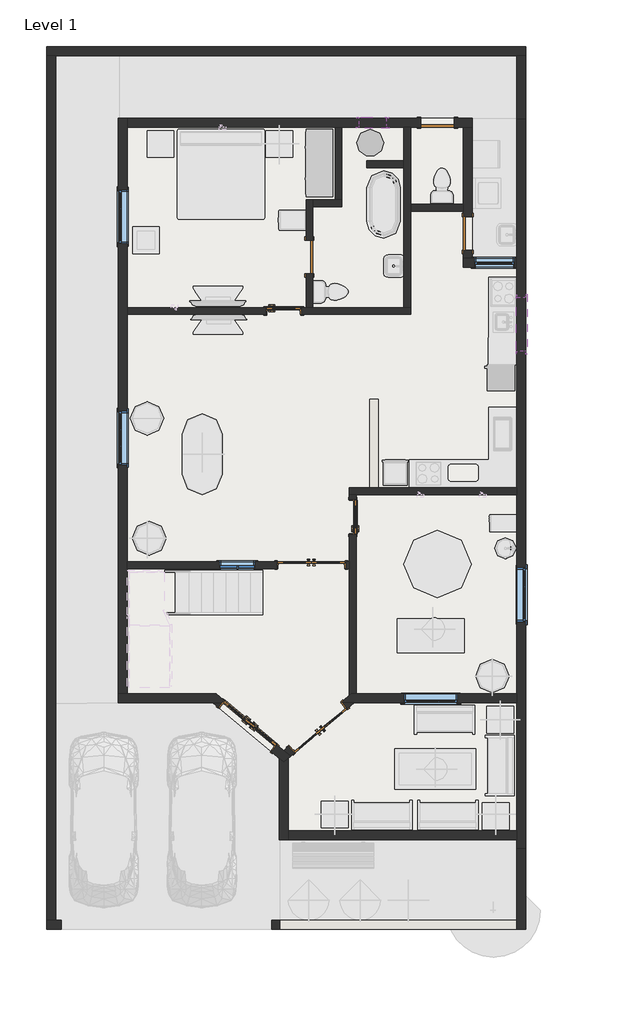
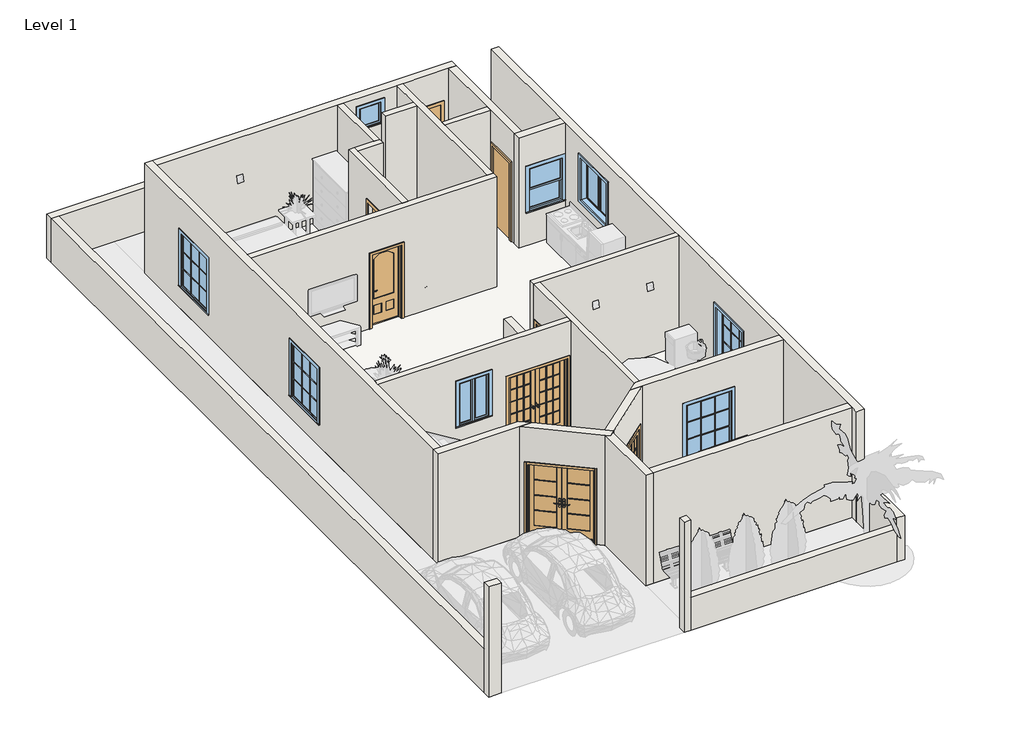
# One storey, part 1 of 2: 29 walls, 8 doors, 8 windows, 1 slab.
"""IFC4 building model written with IfcOpenShell, lengths in millimetres."""

from ifc_helpers import new_model, si_unit, frame, origin, origin_with_axes, place, context, project, spatial, polyline, outline, extrude, faceted_brep, transform, mapped, element, save
from components import door_14b9be53, door_4b146b56, door_b03bd389, door_9d00318c, door_31a77bde, door_e2b13fe9, door_b6acaa4e, window_cfa1ffdd, window_02f8983a, window_0862ab64, window_31198920, window_e41d21a6

model = new_model("IFC4")

# Units and contexts
model_context = context("Model", 3, world=origin())
ifc_project = project(units=[si_unit("LENGTHUNIT", "METRE", prefix="MILLI")], contexts=[model_context])

# Site, building, storey
site = spatial("IfcSite", under=ifc_project)
building = spatial("IfcBuilding", under=site)
storey = spatial("IfcBuildingStorey", under=building, Name="Level 1", Elevation=0.0)

# Doors
placement = place(None, origin())
door_shape = door_14b9be53(model_context)
element("IfcDoor", 1, ObjectType="30\" x 80\"", at=placement, inside=storey, context=model_context, shape_type="MappedRepresentation", body=[
    mapped(door_shape, transform((-5532.7438136, 6064.1316988, 0.0), x_axis=(0.0, -1.0, 0.0), y_axis=(1.0, 0.0, 0.0), z_axis=(0.0, 0.0, 1.0))),
])
door_2_shape = door_4b146b56(model_context)
element("IfcDoor", 2, ObjectType="30\" x 80\"", at=placement, inside=storey, context=model_context, shape_type="MappedRepresentation", body=[
    mapped(door_2_shape, transform((-7101.4900205, 10740.9066988, 0.0), x_axis=(-1.0, 0.0, 0.0), y_axis=(0.0, -1.0, 0.0), z_axis=(0.0, 0.0, 1.0))),
])
door_3_shape = door_b03bd389(model_context)
element("IfcDoor", 3, ObjectType="Door-Exterior-Double-Full Glass-Wood_Clad : 60\" x 80\"", at=placement, inside=storey, context=model_context, shape_type="MappedRepresentation", body=[
    mapped(door_3_shape, transform((-7916.5640809, 1322.8164576, 0.0), x_axis=(0.7664683001194073, -0.6422821380920275, 0.0), y_axis=(0.6422821380920275, 0.7664683001194073, 0.0), z_axis=(0.0, 0.0, 1.0))),
])
door_4_shape = door_9d00318c(model_context)
element("IfcDoor", 4, ObjectType="Door-Interior-Double-Full Glass-Wood : 60\" x 80\"", at=placement, inside=storey, context=model_context, shape_type="MappedRepresentation", body=[
    mapped(door_4_shape, transform((-6321.9607193, 1285.6195575, 0.0), x_axis=(-0.7660444431189786, -0.6427876096865387, 0.0), y_axis=(0.6427876096865387, -0.7660444431189786, 0.0), z_axis=(0.0, 0.0, 1.0))),
])
door_5_shape = door_31a77bde(model_context)
element("IfcDoor", 5, ObjectType="Door-Interior-Double-Full Glass-Wood : 60\" x 80\"", at=placement, inside=storey, context=model_context, shape_type="MappedRepresentation", body=[
    mapped(door_5_shape, transform((-6475.7188136, 4975.1066988, 0.0), x_axis=(1.0, 0.0, 0.0), y_axis=(0.0, 1.0, 0.0), z_axis=(0.0, 0.0, 1.0))),
])
door_6_shape = door_e2b13fe9(model_context)
element("IfcDoor", 6, ObjectType="Single-Flush : 30\" x 84\"", at=placement, inside=storey, context=model_context, shape_type="MappedRepresentation", body=[
    mapped(door_6_shape, transform((-6517.2900205, 11956.9316988, 0.0), x_axis=(0.0, 1.0, 0.0), y_axis=(-1.0, 0.0, 0.0), z_axis=(0.0, 0.0, 1.0))),
])
door_7_shape = door_b6acaa4e(model_context)
element("IfcDoor", 7, ObjectType="Single-Flush : 30\" x 84\"", at=placement, inside=storey, context=model_context, shape_type="MappedRepresentation", body=[
    mapped(door_7_shape, transform((-3614.5602428, 15004.9316988, 0.0), x_axis=(-1.0, 0.0, 0.0), y_axis=(0.0, -1.0, 0.0), z_axis=(0.0, 0.0, 1.0))),
])
element("IfcDoor", 8, ObjectType="Single-Flush : 30\" x 84\"", at=placement, inside=storey, context=model_context, shape_type="MappedRepresentation", body=[
    mapped(door_7_shape, transform((-2928.7602428, 12490.3316988, 0.0), x_axis=(0.0, 1.0, 0.0), y_axis=(-1.0, 0.0, 0.0), z_axis=(0.0, 0.0, 1.0))),
])

# Slab
element("IfcSlab", 9, at=placement, inside=storey, context=model_context, shape_type="SweptSolid", body=[
    extrude(outline(polyline([(-2827.1602428, 15106.5316988), (-2827.1602428, 11931.5316988), (-1607.9602428, 11931.5316988), (-1607.9602428, -1251.0683012), (-7203.0900205, -1251.0683012), (-7203.0900205, 588.2438145), (-8706.1016729, 1847.7316988), (-10853.5602428, 1847.7316988), (-10853.5602428, 15106.5316988), (-2827.1602428, 15106.5316988)])), frame((0.0, 0.0, -323.85), z_axis=(0.0, 0.0, 1.0), x_axis=(1.0, 0.0, 0.0)), (0.0, 0.0, 1.0), 323.85),
])

# Walls
element("IfcWall", 10, ObjectType="Generic - 8\"", at=placement, inside=storey, context=model_context, shape_type="Brep", body=[
    faceted_brep([(-12479.1602428, 16528.9316988, 0.0), (-12275.9602428, 16528.9316988, 0.0), (-1811.1602428, 16528.9316988, 0.0), (-1607.9602428, 16528.9316988, 0.0), (-1607.9602428, 16528.9316988, 1219.2), (-1811.1602428, 16528.9316988, 1219.2), (-12275.9602428, 16528.9316988, 1219.2), (-12479.1602428, 16528.9316988, 1219.2), (-12479.1602428, 16732.1316988, 0.0), (-12479.1602428, 16732.1316988, 1219.2), (-1607.9602428, 16732.1316988, 1219.2), (-1607.9602428, 16732.1316988, 0.0)], [[[0, 1, 2, 3, 4, 5, 6, 7]], [[8, 9, 10, 11]], [[3, 2, 1, 0, 8, 11]], [[7, 6, 5, 4, 10, 9]], [[4, 3, 11, 10]], [[0, 7, 9, 8]]]),
])
element("IfcWall", 11, ObjectType="Generic - 8\"", at=placement, inside=storey, context=model_context, shape_type="SweptSolid", body=[
    extrude(outline(polyline([(-1811.1602428, 15081.1316988), (-1811.1602428, 16528.9316988), (-1607.9602428, 16528.9316988), (-1607.9602428, 15081.1316988), (-1811.1602428, 15081.1316988)])), origin_with_axes(), (0.0, 0.0, 1.0), 1219.2),
])
element("IfcWall", 12, ObjectType="Generic - 8\"", at=placement, inside=storey, context=model_context, shape_type="SweptSolid", body=[
    extrude(outline(polyline([(-7195.9602428, -3079.8683012), (-1811.1602428, -3079.8683012), (-1811.1602428, -3283.0683012), (-7195.9602428, -3283.0683012), (-7195.9602428, -3079.8683012)])), origin_with_axes(), (0.0, 0.0, 1.0), 914.4),
])
element("IfcWall", 13, ObjectType="Generic - 8\"", at=placement, inside=storey, context=model_context, shape_type="SweptSolid", body=[
    extrude(outline(polyline([(-12275.9602428, 16528.9316988), (-12275.9602428, -3079.8683012), (-12479.1602428, -3079.8683012), (-12479.1602428, 16528.9316988), (-12275.9602428, 16528.9316988)])), origin_with_axes(), (0.0, 0.0, 1.0), 1219.2),
])
element("IfcWall", 14, ObjectType="Generic - 8\"", at=placement, inside=storey, context=model_context, shape_type="Brep", body=[
    faceted_brep([(-7203.0900205, 588.2438145, 0.0), (-7203.0900205, -1251.0683012, 0.0), (-7203.0900205, -1251.0683012, 3048.0), (-7203.0900205, 588.2438145, 3048.0), (-6999.8900205, 588.2846184, 0.0), (-6999.8900205, 588.2846184, 3048.0), (-6999.8900205, -1047.8683012, 3048.0), (-6999.8900205, -1251.0683012, 3048.0), (-6999.8900205, -1251.0683012, 0.0), (-6999.8900205, -1047.8683012, 0.0), (-7101.4462872, 503.0687925, 0.0), (-7101.4462872, 503.0687925, 3048.0)], [[[0, 1, 2, 3]], [[4, 5, 6, 7, 8, 9]], [[1, 0, 10, 4, 9, 8]], [[2, 1, 8, 7]], [[0, 3, 11, 10]], [[11, 5, 4, 10]], [[3, 2, 7, 6, 5, 11]]]),
])
element("IfcWall", 15, ObjectType="Generic - 8\"", at=placement, inside=storey, context=model_context, shape_type="SweptSolid", body=[
    extrude(outline(polyline([(-1811.1602428, -1251.0683012), (-6999.8900205, -1251.0683012), (-6999.8900205, -1047.8683012), (-1811.1602428, -1047.8683012), (-1811.1602428, -1251.0683012)])), origin_with_axes(), (0.0, 0.0, 1.0), 3048.0),
])
element("IfcWall", 16, ObjectType="Generic - 8\"", at=placement, inside=storey, context=model_context, shape_type="Brep", body=[
    faceted_brep([(-1811.1602428, 1847.7316988, 0.0), (-1811.1602428, 1847.7316988, 3048.0), (-5498.9394378, 1847.7316988, 3048.0), (-5815.0625194, 1847.7316988, 3048.0), (-5815.0625194, 1847.7316988, 2057.4), (-5765.7511101, 1847.7316988, 2057.4), (-5765.7511101, 1847.7316988, 0.0), (-5498.9394378, 1847.7316988, 0.0), (-4376.5602428, 1847.7316988, 2133.6), (-3157.3602428, 1847.7316988, 2133.6), (-3157.3602428, 1847.7316988, 609.6), (-4376.5602428, 1847.7316988, 609.6), (-1811.1602428, 2050.9316988, 0.0), (-5459.7188136, 2050.9316988, 0.0), (-5572.8981894, 2050.9316988, 0.0), (-5572.8981894, 2050.9316988, 3048.0), (-5459.7188136, 2050.9316988, 3048.0), (-1811.1602428, 2050.9316988, 3048.0), (-4376.5602428, 2050.9316988, 2133.6), (-4376.5602428, 2050.9316988, 609.6), (-3157.3602428, 2050.9316988, 609.6), (-3157.3602428, 2050.9316988, 2133.6), (-5786.1253966, 1872.0128279, 0.0), (-5612.1188136, 2018.0216875, 0.0), (-5786.1253966, 1872.0128279, 2057.4), (-5612.1188136, 2018.0216875, 3048.0)], [[[0, 1, 2, 3, 4, 5, 6, 7], [8, 9, 10, 11]], [[12, 13, 14, 15, 16, 17], [18, 19, 20, 21]], [[14, 13, 12, 0, 7, 6, 22, 23]], [[1, 0, 12, 17]], [[15, 14, 23, 22, 24, 4, 3, 25]], [[24, 5, 4]], [[5, 24, 22, 6]], [[19, 18, 8, 11]], [[20, 19, 11, 10]], [[21, 20, 10, 9]], [[18, 21, 9, 8]], [[3, 2, 1, 17, 16, 15, 25]]]),
])
element("IfcWall", 17, ObjectType="Generic - 8\"", at=placement, inside=storey, context=model_context, shape_type="Brep", body=[
    faceted_brep([(-8706.1016729, 1847.7316988, 3048.0), (-8706.1016729, 1847.7316988, 0.0), (-8587.3763315, 1748.242697, 0.0), (-8587.3763315, 1748.242697, 2057.4), (-7380.3420524, 736.7767859, 2057.4), (-7380.3420524, 736.7767859, 0.0), (-7203.0900205, 588.2438145, 0.0), (-7101.4462872, 503.0687925, 0.0), (-7101.4462872, 503.0687925, 3048.0), (-7203.0900205, 588.2438145, 3048.0), (-6943.3663247, 635.7136307, 3048.0), (-6943.3663247, 635.7136307, 0.0), (-7101.5337538, 768.2541605, 0.0), (-7249.830322, 892.5231445, 0.0), (-7249.830322, 892.5231445, 2057.4), (-8389.7298046, 1847.7316988, 2057.4), (-8389.7298046, 1847.7316988, 3048.0), (-7101.5337538, 768.2541605, 3048.0), (-6999.8900205, 588.2846184, 0.0), (-8504.006923, 1847.7316988, 0.0), (-8504.006923, 1847.7316988, 2057.4), (-6999.8900205, 588.2846184, 3048.0)], [[[0, 1, 2, 3, 4, 5, 6, 7, 8, 9]], [[10, 11, 12, 13, 14, 15, 16, 17]], [[11, 18, 7, 6, 5, 13, 12]], [[2, 1, 19]], [[1, 0, 16, 15, 20, 19]], [[8, 7, 18, 11, 10, 21]], [[4, 14, 13, 5]], [[14, 4, 3, 20, 15]], [[20, 3, 2, 19]], [[0, 9, 8, 21, 10, 17, 16]]]),
])
element("IfcWall", 18, ObjectType="Generic - 8\"", at=placement, inside=storey, context=model_context, shape_type="Brep", body=[
    faceted_brep([(-6943.3663247, 635.7136307, 3048.0), (-6943.3663247, 635.7136307, 0.0), (-6861.8777433, 704.0906693, 0.0), (-6861.8777433, 704.0906693, 2057.4), (-5655.5109543, 1716.3525971, 2057.4), (-5655.5109543, 1716.3525971, 0.0), (-5498.9394378, 1847.7316988, 0.0), (-5498.9394378, 1847.7316988, 3048.0), (-7101.5337538, 768.2541605, 0.0), (-7101.5337538, 768.2541605, 3048.0), (-5815.0625194, 1847.7316988, 3048.0), (-5815.0625194, 1847.7316988, 2057.4), (-6992.4921856, 859.7509002, 2057.4), (-6992.4921856, 859.7509002, 0.0), (-5765.7511101, 1847.7316988, 0.0), (-5765.7511101, 1847.7316988, 2057.4)], [[[0, 1, 2, 3, 4, 5, 6, 7]], [[8, 9, 10, 11, 12, 13]], [[1, 8, 13, 2]], [[6, 5, 14]], [[1, 0, 9, 8]], [[7, 6, 14, 15, 11, 10]], [[12, 3, 2, 13]], [[3, 12, 11, 15, 4]], [[4, 15, 14, 5]], [[0, 7, 10, 9]]]),
])
element("IfcWall", 19, ObjectType="Generic - 8\"", at=placement, inside=storey, context=model_context, shape_type="Brep", body=[
    faceted_brep([(-12148.9602428, -3079.8683012, 0.0), (-12275.9602428, -3079.8683012, 0.0), (-12479.1602428, -3079.8683012, 0.0), (-12479.1602428, -3079.8683012, 1219.2), (-12479.1602428, -3079.8683012, 3048.0), (-12148.9602428, -3079.8683012, 3048.0), (-12148.9602428, -3283.0683012, 0.0), (-12148.9602428, -3283.0683012, 3048.0), (-12479.1602428, -3283.0683012, 3048.0), (-12479.1602428, -3283.0683012, 0.0)], [[[0, 1, 2, 3, 4, 5]], [[6, 7, 8, 9]], [[2, 1, 0, 6, 9]], [[0, 5, 7, 6]], [[4, 3, 2, 9, 8]], [[5, 4, 8, 7]]]),
])
element("IfcWall", 20, ObjectType="Generic - 8\"", at=placement, inside=storey, context=model_context, shape_type="Brep", body=[
    faceted_brep([(-10853.5602428, 1847.7316988, 3048.0), (-10853.5602428, 1847.7316988, 0.0), (-8706.1016729, 1847.7316988, 0.0), (-8504.006923, 1847.7316988, 0.0), (-8504.006923, 1847.7316988, 2057.4), (-8389.7298046, 1847.7316988, 2057.4), (-8389.7298046, 1847.7316988, 3048.0), (-8706.1016729, 1847.7316988, 3048.0), (-8632.2188127, 2050.9316988, 0.0), (-10650.3602428, 2050.9316988, 0.0), (-10853.5602428, 2050.9316988, 0.0), (-10853.5602428, 2050.9316988, 3048.0), (-10650.3602428, 2050.9316988, 3048.0), (-8632.2188127, 2050.9316988, 3048.0), (-8456.864601, 1903.9890555, 0.0), (-8456.864601, 1903.9890555, 2057.4)], [[[0, 1, 2, 3, 4, 5, 6, 7]], [[8, 9, 10, 11, 12, 13]], [[10, 9, 8, 14, 3, 2, 1]], [[8, 13, 6, 5, 15, 14]], [[1, 0, 11, 10]], [[4, 15, 5]], [[15, 4, 3, 14]], [[0, 7, 6, 13, 12, 11]]]),
])
element("IfcWall", 21, ObjectType="Generic - 8\"", at=placement, inside=storey, context=model_context, shape_type="Brep", body=[
    faceted_brep([(-10853.5602428, 15106.5316988, 0.0), (-10853.5602428, 2050.9316988, 0.0), (-10853.5602428, 2050.9316988, 3048.0), (-10853.5602428, 15106.5316988, 3048.0), (-10853.5602428, 8464.4316988, 2133.6), (-10853.5602428, 7245.2316988, 2133.6), (-10853.5602428, 7245.2316988, 609.6), (-10853.5602428, 8464.4316988, 609.6), (-10853.5602428, 13480.9316988, 2133.6), (-10853.5602428, 12261.7316988, 2133.6), (-10853.5602428, 12261.7316988, 609.6), (-10853.5602428, 13480.9316988, 609.6), (-10650.3602428, 15106.5316988, 0.0), (-10650.3602428, 15106.5316988, 3048.0), (-10650.3602428, 14903.3316988, 3048.0), (-10650.3602428, 10813.9316988, 3048.0), (-10650.3602428, 10661.5316988, 3048.0), (-10650.3602428, 5048.1316988, 3048.0), (-10650.3602428, 4895.7316988, 3048.0), (-10650.3602428, 2050.9316988, 3048.0), (-10650.3602428, 2050.9316988, 0.0), (-10650.3602428, 4895.7316988, 0.0), (-10650.3602428, 5048.1316988, 0.0), (-10650.3602428, 10661.5316988, 0.0), (-10650.3602428, 10813.9316988, 0.0), (-10650.3602428, 14903.3316988, 0.0), (-10650.3602428, 8464.4316988, 2133.6), (-10650.3602428, 8464.4316988, 609.6), (-10650.3602428, 7245.2316988, 609.6), (-10650.3602428, 7245.2316988, 2133.6), (-10650.3602428, 13480.9316988, 2133.6), (-10650.3602428, 13480.9316988, 609.6), (-10650.3602428, 12261.7316988, 609.6), (-10650.3602428, 12261.7316988, 2133.6)], [[[0, 1, 2, 3], [4, 5, 6, 7], [8, 9, 10, 11]], [[12, 13, 14, 15, 16, 17, 18, 19, 20, 21, 22, 23, 24, 25], [26, 27, 28, 29], [30, 31, 32, 33]], [[1, 0, 12, 25, 24, 23, 22, 21, 20]], [[2, 1, 20, 19]], [[0, 3, 13, 12]], [[27, 26, 4, 7]], [[28, 27, 7, 6]], [[29, 28, 6, 5]], [[26, 29, 5, 4]], [[31, 30, 8, 11]], [[32, 31, 11, 10]], [[33, 32, 10, 9]], [[30, 33, 9, 8]], [[3, 2, 19, 18, 17, 16, 15, 14, 13]]]),
])
element("IfcWall", 22, ObjectType="Generic - 8\"", at=placement, inside=storey, context=model_context, shape_type="Brep", body=[
    faceted_brep([(-3030.3602428, 11931.5316988, 0.0), (-3030.3602428, 11931.5316988, 3048.0), (-3030.3602428, 12998.3316988, 3048.0), (-3030.3602428, 13150.7316988, 3048.0), (-3030.3602428, 14903.3316988, 3048.0), (-3030.3602428, 14903.3316988, 0.0), (-3030.3602428, 13150.7316988, 0.0), (-3030.3602428, 12998.3316988, 0.0), (-3030.3602428, 12871.3316988, 0.0), (-3030.3602428, 12871.3316988, 2133.6), (-3030.3602428, 12109.3316988, 2133.6), (-3030.3602428, 12109.3316988, 0.0), (-2827.1602428, 11931.5316988, 3048.0), (-2827.1602428, 11931.5316988, 0.0), (-2827.1602428, 12109.3316988, 0.0), (-2827.1602428, 12109.3316988, 2133.6), (-2827.1602428, 12871.3316988, 2133.6), (-2827.1602428, 12871.3316988, 0.0), (-2827.1602428, 14903.3316988, 0.0), (-2827.1602428, 14903.3316988, 3048.0)], [[[0, 1, 2, 3, 4, 5, 6, 7, 8, 9, 10, 11]], [[12, 13, 14, 15, 16, 17, 18, 19]], [[13, 0, 11, 14]], [[5, 18, 17, 8, 7, 6]], [[1, 0, 13, 12]], [[5, 4, 19, 18]], [[16, 9, 8, 17]], [[9, 16, 15, 10]], [[10, 15, 14, 11]], [[4, 3, 2, 1, 12, 19]]]),
])
element("IfcWall", 23, ObjectType="Generic - 8\"", at=placement, inside=storey, context=model_context, shape_type="Brep", body=[
    faceted_brep([(-3995.5602428, 15106.5316988, 2133.6), (-3995.5602428, 15106.5316988, 0.0), (-10650.3602428, 15106.5316988, 0.0), (-10650.3602428, 15106.5316988, 3048.0), (-2827.1602428, 15106.5316988, 3048.0), (-2827.1602428, 15106.5316988, 0.0), (-3233.5602428, 15106.5316988, 0.0), (-3233.5602428, 15106.5316988, 2133.6), (-5383.4251316, 15106.5316988, 2768.6), (-5383.4251316, 15106.5316988, 2159.0), (-4773.8251316, 15106.5316988, 2159.0), (-4773.8251316, 15106.5316988, 2768.6), (-10650.3602428, 14903.3316988, 0.0), (-5933.0900205, 14903.3316988, 0.0), (-5780.6900205, 14903.3316988, 0.0), (-4376.5602428, 14903.3316988, 0.0), (-4224.1602428, 14903.3316988, 0.0), (-3995.5602428, 14903.3316988, 0.0), (-3995.5602428, 14903.3316988, 2133.6), (-3233.5602428, 14903.3316988, 2133.6), (-3233.5602428, 14903.3316988, 0.0), (-3030.3602428, 14903.3316988, 0.0), (-2827.1602428, 14903.3316988, 0.0), (-2827.1602428, 14903.3316988, 3048.0), (-3030.3602428, 14903.3316988, 3048.0), (-4224.1602428, 14903.3316988, 3048.0), (-4376.5602428, 14903.3316988, 3048.0), (-5780.6900205, 14903.3316988, 3048.0), (-5933.0900205, 14903.3316988, 3048.0), (-10650.3602428, 14903.3316988, 3048.0), (-5383.4251316, 14903.3316988, 2768.6), (-4773.8251316, 14903.3316988, 2768.6), (-4773.8251316, 14903.3316988, 2159.0), (-5383.4251316, 14903.3316988, 2159.0)], [[[0, 1, 2, 3, 4, 5, 6, 7], [8, 9, 10, 11]], [[12, 13, 14, 15, 16, 17, 18, 19, 20, 21, 22, 23, 24, 25, 26, 27, 28, 29], [30, 31, 32, 33]], [[6, 5, 22, 21, 20]], [[2, 1, 17, 16, 15, 14, 13, 12]], [[3, 2, 12, 29]], [[5, 4, 23, 22]], [[18, 17, 1, 0]], [[19, 18, 0, 7]], [[20, 19, 7, 6]], [[4, 3, 29, 28, 27, 26, 25, 24, 23]], [[9, 8, 30, 33]], [[10, 9, 33, 32]], [[11, 10, 32, 31]], [[8, 11, 31, 30]]]),
])
element("IfcWall", 24, ObjectType="Generic - 8\"", at=placement, inside=storey, context=model_context, shape_type="Brep", body=[
    faceted_brep([(-1811.1602428, 11931.5316988, 0.0), (-2827.1602428, 11931.5316988, 0.0), (-3030.3602428, 11931.5316988, 0.0), (-3030.3602428, 11931.5316988, 3048.0), (-2827.1602428, 11931.5316988, 3048.0), (-1811.1602428, 11931.5316988, 3048.0), (-2776.3602428, 11931.5316988, 2133.6), (-2776.3602428, 11931.5316988, 914.4), (-1861.9602428, 11931.5316988, 914.4), (-1861.9602428, 11931.5316988, 2133.6), (-1811.1602428, 11728.3316988, 0.0), (-1811.1602428, 11728.3316988, 3048.0), (-3030.3602428, 11728.3316988, 3048.0), (-3030.3602428, 11728.3316988, 0.0), (-2776.3602428, 11728.3316988, 2133.6), (-1861.9602428, 11728.3316988, 2133.6), (-1861.9602428, 11728.3316988, 914.4), (-2776.3602428, 11728.3316988, 914.4)], [[[0, 1, 2, 3, 4, 5], [6, 7, 8, 9]], [[10, 11, 12, 13], [14, 15, 16, 17]], [[2, 1, 0, 10, 13]], [[0, 5, 11, 10]], [[3, 2, 13, 12]], [[7, 6, 14, 17]], [[8, 7, 17, 16]], [[9, 8, 16, 15]], [[6, 9, 15, 14]], [[5, 4, 3, 12, 11]]]),
])
element("IfcWall", 25, ObjectType="Generic - 8\"", at=placement, inside=storey, context=model_context, shape_type="Brep", body=[
    faceted_brep([(-7195.9602428, -3079.8683012, 0.0), (-7373.7602428, -3079.8683012, 0.0), (-7373.7602428, -3079.8683012, 3048.0), (-7195.9602428, -3079.8683012, 3048.0), (-7195.9602428, -3079.8683012, 914.4), (-7195.9602428, -3283.0683012, 0.0), (-7195.9602428, -3283.0683012, 914.4), (-7195.9602428, -3283.0683012, 3048.0), (-7373.7602428, -3283.0683012, 3048.0), (-7373.7602428, -3283.0683012, 0.0)], [[[0, 1, 2, 3, 4]], [[5, 6, 7, 8, 9]], [[1, 0, 5, 9]], [[2, 1, 9, 8]], [[0, 4, 3, 7, 6, 5]], [[3, 2, 8, 7]]]),
])
element("IfcWall", 26, ObjectType="Generic - 8\"", at=placement, inside=storey, context=model_context, shape_type="Brep", body=[
    faceted_brep([(-1811.1602428, -1454.2683012, 0.0), (-1811.1602428, -3079.8683012, 0.0), (-1811.1602428, -3283.0683012, 0.0), (-1811.1602428, -3283.0683012, 914.4), (-1811.1602428, -3283.0683012, 1219.2), (-1811.1602428, -1454.2683012, 1219.2), (-1607.9602428, -1454.2683012, 0.0), (-1607.9602428, -1454.2683012, 1219.2), (-1607.9602428, -3283.0683012, 1219.2), (-1607.9602428, -3283.0683012, 0.0)], [[[0, 1, 2, 3, 4, 5]], [[6, 7, 8, 9]], [[2, 1, 0, 6, 9]], [[5, 4, 8, 7]], [[0, 5, 7, 6]], [[4, 3, 2, 9, 8]]]),
])
element("IfcWall", 27, ObjectType="Generic - 8\"", at=placement, inside=storey, context=model_context, shape_type="Brep", body=[
    faceted_brep([(-1811.1602428, 15081.1316988, 0.0), (-1811.1602428, 11931.5316988, 0.0), (-1811.1602428, 11728.3316988, 0.0), (-1811.1602428, 6724.5316988, 0.0), (-1811.1602428, 6572.1316988, 0.0), (-1811.1602428, 2050.9316988, 0.0), (-1811.1602428, 1847.7316988, 0.0), (-1811.1602428, -1047.8683012, 0.0), (-1811.1602428, -1251.0683012, 0.0), (-1811.1602428, -1454.2683012, 0.0), (-1811.1602428, -1454.2683012, 1219.2), (-1811.1602428, -1454.2683012, 3048.0), (-1811.1602428, -1251.0683012, 3048.0), (-1811.1602428, -1047.8683012, 3048.0), (-1811.1602428, 1847.7316988, 3048.0), (-1811.1602428, 2050.9316988, 3048.0), (-1811.1602428, 6572.1316988, 3048.0), (-1811.1602428, 6724.5316988, 3048.0), (-1811.1602428, 11728.3316988, 3048.0), (-1811.1602428, 11931.5316988, 3048.0), (-1811.1602428, 15081.1316988, 3048.0), (-1811.1602428, 15081.1316988, 1219.2), (-1811.1602428, 3689.2316988, 2133.6), (-1811.1602428, 3689.2316988, 609.6), (-1811.1602428, 4908.4316988, 609.6), (-1811.1602428, 4908.4316988, 2133.6), (-1811.1602428, 9823.3316988, 2540.0), (-1811.1602428, 9823.3316988, 1320.8), (-1811.1602428, 11042.5316988, 1320.8), (-1811.1602428, 11042.5316988, 2540.0), (-1607.9602428, 15081.1316988, 0.0), (-1607.9602428, 15081.1316988, 1219.2), (-1607.9602428, 15081.1316988, 3048.0), (-1607.9602428, -1454.2683012, 3048.0), (-1607.9602428, -1454.2683012, 1219.2), (-1607.9602428, -1454.2683012, 0.0), (-1607.9602428, 3689.2316988, 2133.6), (-1607.9602428, 4908.4316988, 2133.6), (-1607.9602428, 4908.4316988, 609.6), (-1607.9602428, 3689.2316988, 609.6), (-1607.9602428, 9823.3316988, 2540.0), (-1607.9602428, 11042.5316988, 2540.0), (-1607.9602428, 11042.5316988, 1320.8), (-1607.9602428, 9823.3316988, 1320.8)], [[[0, 1, 2, 3, 4, 5, 6, 7, 8, 9, 10, 11, 12, 13, 14, 15, 16, 17, 18, 19, 20, 21], [22, 23, 24, 25], [26, 27, 28, 29]], [[30, 31, 32, 33, 34, 35], [36, 37, 38, 39], [40, 41, 42, 43]], [[9, 8, 7, 6, 5, 4, 3, 2, 1, 0, 30, 35]], [[11, 10, 9, 35, 34, 33]], [[0, 21, 20, 32, 31, 30]], [[23, 22, 36, 39]], [[24, 23, 39, 38]], [[25, 24, 38, 37]], [[22, 25, 37, 36]], [[27, 26, 40, 43]], [[28, 27, 43, 42]], [[29, 28, 42, 41]], [[26, 29, 41, 40]], [[20, 19, 18, 17, 16, 15, 14, 13, 12, 11, 33, 32]]]),
])
element("IfcWall", 28, ObjectType="Generic - 8\"", at=placement, inside=storey, context=model_context, shape_type="SweptSolid", body=[
    extrude(outline(polyline([(-4951.7188136, 8731.1316988), (-4951.7188136, 6724.5316988), (-5154.9188136, 6724.5316988), (-5154.9188136, 8731.1316988), (-4951.7188136, 8731.1316988)])), origin_with_axes(), (0.0, 0.0, 1.0), 609.6),
])
element("IfcWall", 29, ObjectType="INNER WALL", at=placement, inside=storey, context=model_context, shape_type="Brep", body=[
    faceted_brep([(-1811.1602428, 6724.5316988, 0.0), (-4951.7188136, 6724.5316988, 0.0), (-5154.9188136, 6724.5316988, 0.0), (-5612.1188136, 6724.5316988, 0.0), (-5612.1188136, 6724.5316988, 3048.0), (-1811.1602428, 6724.5316988, 3048.0), (-1811.1602428, 6572.1316988, 0.0), (-1811.1602428, 6572.1316988, 3048.0), (-5459.7188136, 6572.1316988, 3048.0), (-5612.1188136, 6572.1316988, 3048.0), (-5612.1188136, 6572.1316988, 0.0), (-5459.7188136, 6572.1316988, 0.0)], [[[0, 1, 2, 3, 4, 5]], [[6, 7, 8, 9, 10, 11]], [[3, 2, 1, 0, 6, 11, 10]], [[0, 5, 7, 6]], [[4, 3, 10, 9]], [[5, 4, 9, 8, 7]]]),
])
element("IfcWall", 30, ObjectType="INNER WALL", at=placement, inside=storey, context=model_context, shape_type="Brep", body=[
    faceted_brep([(-5459.7188136, 2050.9316988, 3048.0), (-5459.7188136, 2050.9316988, 0.0), (-5459.7188136, 5657.7316988, 0.0), (-5459.7188136, 5657.7316988, 2057.4), (-5459.7188136, 6470.5316988, 2057.4), (-5459.7188136, 6470.5316988, 0.0), (-5459.7188136, 6572.1316988, 0.0), (-5459.7188136, 6572.1316988, 3048.0), (-5612.1188136, 2018.0216875, 0.0), (-5612.1188136, 2018.0216875, 3048.0), (-5612.1188136, 4895.7316988, 3048.0), (-5612.1188136, 5048.1316988, 3048.0), (-5612.1188136, 6572.1316988, 3048.0), (-5612.1188136, 6572.1316988, 0.0), (-5612.1188136, 6470.5316988, 0.0), (-5612.1188136, 6470.5316988, 2057.4), (-5612.1188136, 5657.7316988, 2057.4), (-5612.1188136, 5657.7316988, 0.0), (-5612.1188136, 5048.1316988, 0.0), (-5612.1188136, 4895.7316988, 0.0), (-5572.8981894, 2050.9316988, 0.0), (-5572.8981894, 2050.9316988, 3048.0)], [[[0, 1, 2, 3, 4, 5, 6, 7]], [[8, 9, 10, 11, 12, 13, 14, 15, 16, 17, 18, 19]], [[1, 20, 8, 19, 18, 17, 2]], [[13, 6, 5, 14]], [[1, 0, 21, 20]], [[9, 8, 20, 21]], [[7, 6, 13, 12]], [[16, 3, 2, 17]], [[3, 16, 15, 4]], [[4, 15, 14, 5]], [[0, 7, 12, 11, 10, 9, 21]]]),
])
element("IfcWall", 31, ObjectType="INNER WALL", at=placement, inside=storey, context=model_context, shape_type="Brep", body=[
    faceted_brep([(-10650.3602428, 10661.5316988, 3048.0), (-10650.3602428, 10661.5316988, 0.0), (-7507.8900205, 10661.5316988, 0.0), (-7507.8900205, 10661.5316988, 2057.4), (-6695.0900205, 10661.5316988, 2057.4), (-6695.0900205, 10661.5316988, 0.0), (-4224.1602428, 10661.5316988, 0.0), (-4224.1602428, 10661.5316988, 3048.0), (-10650.3602428, 10813.9316988, 0.0), (-10650.3602428, 10813.9316988, 3048.0), (-6593.4900205, 10813.9316988, 3048.0), (-6441.0900205, 10813.9316988, 3048.0), (-4376.5602428, 10813.9316988, 3048.0), (-4224.1602428, 10813.9316988, 3048.0), (-4224.1602428, 10813.9316988, 0.0), (-4376.5602428, 10813.9316988, 0.0), (-6441.0900205, 10813.9316988, 0.0), (-6593.4900205, 10813.9316988, 0.0), (-6695.0900205, 10813.9316988, 0.0), (-6695.0900205, 10813.9316988, 2057.4), (-7507.8900205, 10813.9316988, 2057.4), (-7507.8900205, 10813.9316988, 0.0)], [[[0, 1, 2, 3, 4, 5, 6, 7]], [[8, 9, 10, 11, 12, 13, 14, 15, 16, 17, 18, 19, 20, 21]], [[1, 8, 21, 2]], [[14, 6, 5, 18, 17, 16, 15]], [[1, 0, 9, 8]], [[7, 6, 14, 13]], [[20, 3, 2, 21]], [[3, 20, 19, 4]], [[4, 19, 18, 5]], [[0, 7, 13, 12, 11, 10, 9]]]),
])
element("IfcWall", 32, ObjectType="INNER WALL", at=placement, inside=storey, context=model_context, shape_type="Brep", body=[
    faceted_brep([(-4224.1602428, 10813.9316988, 0.0), (-4224.1602428, 12998.3316988, 0.0), (-4224.1602428, 13150.7316988, 0.0), (-4224.1602428, 14903.3316988, 0.0), (-4224.1602428, 14903.3316988, 3048.0), (-4224.1602428, 13150.7316988, 3048.0), (-4224.1602428, 12998.3316988, 3048.0), (-4224.1602428, 10813.9316988, 3048.0), (-4376.5602428, 10813.9316988, 0.0), (-4376.5602428, 10813.9316988, 3048.0), (-4376.5602428, 13988.9316988, 3048.0), (-4376.5602428, 14141.3316988, 3048.0), (-4376.5602428, 14903.3316988, 3048.0), (-4376.5602428, 14903.3316988, 0.0), (-4376.5602428, 14141.3316988, 0.0), (-4376.5602428, 13988.9316988, 0.0)], [[[0, 1, 2, 3, 4, 5, 6, 7]], [[8, 9, 10, 11, 12, 13, 14, 15]], [[3, 2, 1, 0, 8, 15, 14, 13]], [[0, 7, 9, 8]], [[4, 3, 13, 12]], [[7, 6, 5, 4, 12, 11, 10, 9]]]),
])
element("IfcWall", 33, ObjectType="INNER WALL", at=placement, inside=storey, context=model_context, shape_type="SweptSolid", body=[
    extrude(outline(polyline([(3048.0, -10650.3602428), (0.0, -10650.3602428), (0.0, -7263.1188136), (2057.4, -7263.1188136), (2057.4, -5688.3188136), (0.0, -5688.3188136), (0.0, -5612.1188136), (3048.0, -5612.1188136), (3048.0, -10650.3602428)]), holes=[polyline([(2362.2, -8558.5188136), (2362.2, -7745.7188136), (1143.0, -7745.7188136), (1143.0, -8558.5188136), (2362.2, -8558.5188136)])]), frame((0.0, 4895.7316988, 0.0), z_axis=(0.0, 1.0, 0.0), x_axis=(0.0, 0.0, 1.0)), (0.0, 0.0, 1.0), 152.4),
])
element("IfcWall", 34, ObjectType="INNER WALL", at=placement, inside=storey, context=model_context, shape_type="Brep", body=[
    faceted_brep([(-6441.0900205, 12337.9316988, 2133.6), (-6441.0900205, 12337.9316988, 0.0), (-6441.0900205, 13099.9316988, 0.0), (-6441.0900205, 13252.3316988, 0.0), (-6441.0900205, 13252.3316988, 3048.0), (-6441.0900205, 13099.9316988, 3048.0), (-6441.0900205, 10813.9316988, 3048.0), (-6441.0900205, 10813.9316988, 0.0), (-6441.0900205, 11575.9316988, 0.0), (-6441.0900205, 11575.9316988, 2133.6), (-6593.4900205, 13252.3316988, 0.0), (-6593.4900205, 12337.9316988, 0.0), (-6593.4900205, 12337.9316988, 2133.6), (-6593.4900205, 11575.9316988, 2133.6), (-6593.4900205, 11575.9316988, 0.0), (-6593.4900205, 10813.9316988, 0.0), (-6593.4900205, 10813.9316988, 3048.0), (-6593.4900205, 13252.3316988, 3048.0)], [[[0, 1, 2, 3, 4, 5, 6, 7, 8, 9]], [[10, 11, 12, 13, 14, 15, 16, 17]], [[8, 7, 15, 14]], [[3, 2, 1, 11, 10]], [[7, 6, 16, 15]], [[4, 3, 10, 17]], [[12, 11, 1, 0]], [[13, 12, 0, 9]], [[14, 13, 9, 8]], [[6, 5, 4, 17, 16]]]),
])
element("IfcWall", 35, ObjectType="INNER WALL", at=placement, inside=storey, context=model_context, shape_type="Brep", body=[
    faceted_brep([(-6441.0900205, 13099.9316988, 0.0), (-5780.6900205, 13099.9316988, 0.0), (-5780.6900205, 13099.9316988, 3048.0), (-6441.0900205, 13099.9316988, 3048.0), (-6441.0900205, 13252.3316988, 0.0), (-6441.0900205, 13252.3316988, 3048.0), (-5933.0900205, 13252.3316988, 3048.0), (-5780.6900205, 13252.3316988, 3048.0), (-5780.6900205, 13252.3316988, 0.0), (-5933.0900205, 13252.3316988, 0.0)], [[[0, 1, 2, 3]], [[4, 5, 6, 7, 8, 9]], [[1, 0, 4, 9, 8]], [[2, 1, 8, 7]], [[0, 3, 5, 4]], [[3, 2, 7, 6, 5]]]),
])
element("IfcWall", 36, ObjectType="INNER WALL", at=placement, inside=storey, context=model_context, shape_type="SweptSolid", body=[
    extrude(outline(polyline([(-5780.6900205, 14903.3316988), (-5780.6900205, 13252.3316988), (-5933.0900205, 13252.3316988), (-5933.0900205, 14903.3316988), (-5780.6900205, 14903.3316988)])), origin_with_axes(), (0.0, 0.0, 1.0), 3048.0),
])
element("IfcWall", 37, ObjectType="INNER WALL", at=placement, inside=storey, context=model_context, shape_type="SweptSolid", body=[
    extrude(outline(polyline([(-4224.1602428, 13150.7316988), (-3030.3602428, 13150.7316988), (-3030.3602428, 12998.3316988), (-4224.1602428, 12998.3316988), (-4224.1602428, 13150.7316988)])), origin_with_axes(), (0.0, 0.0, 1.0), 3048.0),
])
element("IfcWall", 38, ObjectType="INNER WALL", at=placement, inside=storey, context=model_context, shape_type="SweptSolid", body=[
    extrude(outline(polyline([(-5214.7602428, 14141.3316988), (-4376.5602428, 14141.3316988), (-4376.5602428, 13988.9316988), (-5214.7602428, 13988.9316988), (-5214.7602428, 14141.3316988)])), origin_with_axes(), (0.0, 0.0, 1.0), 3048.0),
])

# Windows
window_shape = window_cfa1ffdd(model_context)
element("IfcWindow", 39, ObjectType="Casement 3x3 with Trim : 48\" x 60\"", at=placement, inside=storey, context=model_context, shape_type="MappedRepresentation", body=[
    mapped(window_shape, transform((-3766.9602428, 1949.3316988, 0.0), x_axis=(-1.0, 0.0, 0.0), y_axis=(0.0, -1.0, 0.0), z_axis=(0.0, 0.0, 1.0))),
])
element("IfcWindow", 40, ObjectType="Casement 3x3 with Trim : 48\" x 60\"", at=placement, inside=storey, context=model_context, shape_type="MappedRepresentation", body=[
    mapped(window_shape, transform((-10751.9602428, 7854.8316988, 0.0), x_axis=(0.0, 1.0, 0.0), y_axis=(-1.0, 0.0, 0.0), z_axis=(0.0, 0.0, 1.0))),
])
element("IfcWindow", 41, ObjectType="Casement 3x3 with Trim : 48\" x 60\"", at=placement, inside=storey, context=model_context, shape_type="MappedRepresentation", body=[
    mapped(window_shape, transform((-10751.9602428, 12871.3316988, 0.0), x_axis=(0.0, 1.0, 0.0), y_axis=(-1.0, 0.0, 0.0), z_axis=(0.0, 0.0, 1.0))),
])
element("IfcWindow", 42, ObjectType="Casement 3x3 with Trim : 48\" x 60\"", at=placement, inside=storey, context=model_context, shape_type="MappedRepresentation", body=[
    mapped(window_shape, transform((-1709.5602428, 4298.8316988, 0.0), x_axis=(0.0, -1.0, 0.0), y_axis=(1.0, 0.0, 0.0), z_axis=(0.0, 0.0, 1.0))),
])
window_2_shape = window_02f8983a(model_context)
element("IfcWindow", 43, ObjectType="Casement Dbl with Trim : 32\" x 48\"", at=placement, inside=storey, context=model_context, shape_type="MappedRepresentation", body=[
    mapped(window_2_shape, transform((-8152.1188136, 4990.9816988, 228.6), x_axis=(-1.0, 0.0, 0.0), y_axis=(0.0, -1.0, 0.0), z_axis=(0.0, 0.0, 1.0))),
])
window_3_shape = window_0862ab64(model_context)
element("IfcWindow", 44, ObjectType="Casement Dbl with Trim : 48\" x 48\"", at=placement, inside=storey, context=model_context, shape_type="MappedRepresentation", body=[
    mapped(window_3_shape, transform((-1728.6102428, 10432.9316988, 406.4), x_axis=(0.0, -1.0, 0.0), y_axis=(1.0, 0.0, 0.0), z_axis=(0.0, 0.0, 1.0))),
])
window_4_shape = window_31198920(model_context)
element("IfcWindow", 45, ObjectType="Double Hung with Trim : 36\" x 48\"", at=placement, inside=storey, context=model_context, shape_type="MappedRepresentation", body=[
    mapped(window_4_shape, transform((-2319.1602428, 11829.9316988, 0.0), x_axis=(-1.0, 0.0, 0.0), y_axis=(0.0, -1.0, 0.0), z_axis=(0.0, 0.0, 1.0))),
])
window_5_shape = window_e41d21a6(model_context)
element("IfcWindow", 46, ObjectType="Transom with Trim : 24\" x 24\"", at=placement, inside=storey, context=model_context, shape_type="MappedRepresentation", body=[
    mapped(window_5_shape, transform((-5116.7251316, 15004.9316988, 0.0), x_axis=(-1.0, 0.0, 0.0), y_axis=(0.0, -1.0, 0.0), z_axis=(0.0, 0.0, 1.0))),
])

save(model, "model.ifc")

# Revit data of these elements
# Type "30\" x 80\""
#   Type Mark = "9"
#   Assembly Code = "B2030100"
#   Analytic Construction = "French door, wood frame with single glass"
#   Threshold Offset [instance default] = 0' - 0 1/2"
#   Thickness = 0' - 1 3/8"
#   Thermal Resistance (R) = 1.0696 (h·ft²·°F)/BTU
#   Swing Angle [instance default] = 90.00°
#   Stiles = 0' - 4 3/4"
#   Rough Width = 2' - 8"
#   Rough Height = 6' - 9"
#   Radius = 1' - 1.00625"
#   Lock Rail = 0' - 7 1/8"
#   Height = 6' - 8"
#   Width = 2' - 6"
#   Heat Transfer Coefficient (U) = 0.9350 BTU/(h·ft²·°F)
#   Door Offset [instance default] = 0' - 0"
#   Bottom Rail = 0' - 9 1/2"
#   Threshold [instance default] = yes
#   Function = 1
#   Exterior Trim [instance default] = yes
#   Trim Material = Cherry
#   Threshold Material = Cherry
#   Panel Material = Cherry
#   Glazing = Glass
#   Frame Material = Cherry
#   Door Handle Material = Aluminum
#   Visual Light Transmittance = 0
#   Solar Heat Gain Coefficient = 0
#   Wall Closure = (empty or 0)
#   Construction Type = (empty or 0)
# Type "Door-Exterior-Double-Full Glass-Wood_Clad : 60\" x 80\""
#   Type Mark = "8"
#   Assembly Code = "B2030100"
#   Analytic Construction = "French door, wood frame with double glass"
#   Top Rail = 0' - 4 11/16"
#   Threshold Offset [instance default] = 0' - 0 1/2"
#   Thickness = 0' - 1 3/8"
#   Thermal Resistance (R) = 1.9158 (h·ft²·°F)/BTU
#   Swing Angle [instance default] = 90.00°
#   Stiles = 0' - 4 3/4"
#   Rough Width = 5' - 2"
#   Rough Height = 6' - 9"
#   Panel Width = 2' - 6"
#   Door Offset [instance default] = 0' - 0"
#   Height = 6' - 8"
#   Width = 5' - 0"
#   Heat Transfer Coefficient (U) = 0.5220 BTU/(h·ft²·°F)
#   Bottom Rail = 0' - 9 1/8"
#   Exterior Trim [instance default] = yes
#   Threshold [instance default] = yes
#   Show Grill [instance default] = yes
#   Function = 1
#   Trim Material = Cherry
#   Threshold Material = Cherry
#   Panel Material = Cherry
#   Glazing = Glass
#   Frame Material = Cherry
#   Door Handle Material = Aluminum
#   Visual Light Transmittance = 0
#   Solar Heat Gain Coefficient = 0
#   Wall Closure = (empty or 0)
#   Construction Type = (empty or 0)
# Type "Door-Interior-Double-Full Glass-Wood : 60\" x 80\""
#   Type Mark = "10"
#   Assembly Code = "C1020300"
#   Analytic Construction = "French door, wood frame with single glass"
#   Top Rail = 0' - 4 11/16"
#   Thickness = 0' - 1 3/8"
#   Thermal Resistance (R) = 1.0696 (h·ft²·°F)/BTU
#   Swing Angle [instance default] = 90.00°
#   Stiles = 0' - 4 3/4"
#   Rough Width = 5' - 2"
#   Rough Height = 6' - 9"
#   Panel Width = 2' - 6"
#   Height = 6' - 8"
#   Width = 5' - 0"
#   Heat Transfer Coefficient (U) = 0.9350 BTU/(h·ft²·°F)
#   Bottom Rail = 0' - 9 1/8"
#   Show Grill [instance default] = yes
#   Trim Material = Cherry
#   Panel Material = Cherry
#   Frame Material = Cherry
#   Door Handle Material = Aluminum
#   Visual Light Transmittance = 0
#   Solar Heat Gain Coefficient = 0
#   Wall Closure = (empty or 0)
#   Function = (empty or 0)
# Type "Single-Flush : 30\" x 84\""
#   Type Mark = "1"
#   Construction Type Id = "MDOOR"
#   Assembly Code = "C1020"
#   Analytic Construction = "Metal"
#   Thickness = 0' - 2"
#   Heat Transfer Coefficient (U) = 0.651978 BTU/(h·ft²·°F)
#   Height = 7' - 0"
#   Trim Projection Ext = 0' - 1"
#   Trim Projection Int = 0' - 1"
#   Trim Width = 0' - 3"
#   Width = 2' - 6"
#   Define Thermal Properties by = 1
#   Door Material = Door - Panel
#   Frame Material = Door - Frame
#   Visual Light Transmittance = 0
#   Solar Heat Gain Coefficient = 0
#   Function = (empty or 0)
#   Wall Closure = (empty or 0)
# Type
#   Assembly Code = "B1010"
#   Function = 0
#   Layers, outside or top first: 0' - 0 1/8" "Carpet (1)" (function 4); 0' - 0 3/4" "Plywood, Sheathing" (function 1); 0' - 11 7/8" "Structure, Wood Joist/Rafter Layer" (function 1)
# Type "Generic - 8\""
#   Assembly Code = "B2010"
#   Layers, outside or top first: 0' - 8" "Brick, Common" (function 1)
# Type "INNER WALL"
#   Assembly Code = "B2010"
#   Layers, outside or top first: 0' - 6" "Brick, Soldier Course" (function 1)
# Type "Casement 3x3 with Trim : 48\" x 60\""
#   Type Mark = "11"
#   Construction Type Id = "GSP4R"
#   Assembly Code = "B2020100"
#   Analytic Construction = "1/8 in Pilkington single glazing"
#   Visual Light Transmittance = 0.9
#   Solar Heat Gain Coefficient = 0.78
#   Heat Transfer Coefficient (U) = 0.6496 BTU/(h·ft²·°F)
#   Height = 5' - 0"
#   Default Sill Height = 2' - 0"
#   Trim Projection - Ext. = 0' - 0 1/2"
#   Trim Projection - Int. = 0' - 0 3/4"
#   Trim Width - Exterior = 0' - 3 1/2"
#   Trim Width - Interior = 0' - 3 1/2"
#   Width = 4' - 0"
#   Window Inset = 0' - 0 3/4"
#   Define Thermal Properties by = 1
#   Glass Pane Material = Glass
#   Sash Material = Sash
#   Trim Exterior Material = Trim
#   Trim Interior Material = Trim
#   Wall Closure = (empty or 0)
# Type "Casement Dbl with Trim : 32\" x 48\""
#   Type Mark = "15"
#   Construction Type Id = "GSP4R"
#   Assembly Code = "B2020100"
#   Analytic Construction = "1/8 in Pilkington single glazing"
#   Visual Light Transmittance = 0.9
#   Solar Heat Gain Coefficient = 0.78
#   Heat Transfer Coefficient (U) = 0.6496 BTU/(h·ft²·°F)
#   Height = 4' - 0"
#   Default Sill Height = 3' - 0"
#   Trim Projection - Ext. = 0' - 0 1/2"
#   Trim Projection - Int. = 0' - 0 3/4"
#   Trim Width - Exterior = 0' - 3 1/2"
#   Trim Width - Interior = 0' - 3 1/2"
#   Width = 2' - 8"
#   Window Inset = 0' - 0 3/4"
#   Define Thermal Properties by = 1
#   Glass Pane Material = Glass
#   Sash Material = Sash
#   Trim Exterior Material = Trim
#   Trim Interior Material = Trim
#   Wall Closure = (empty or 0)
# Type "Casement Dbl with Trim : 48\" x 48\""
#   Type Mark = "13"
#   Construction Type Id = "GSP4R"
#   Assembly Code = "B2020100"
#   Analytic Construction = "1/8 in Pilkington single glazing"
#   Visual Light Transmittance = 0.9
#   Solar Heat Gain Coefficient = 0.78
#   Heat Transfer Coefficient (U) = 0.6496 BTU/(h·ft²·°F)
#   Height = 4' - 0"
#   Default Sill Height = 3' - 0"
#   Trim Projection - Ext. = 0' - 0 1/2"
#   Trim Projection - Int. = 0' - 0 3/4"
#   Trim Width - Exterior = 0' - 3 1/2"
#   Trim Width - Interior = 0' - 3 1/2"
#   Width = 4' - 0"
#   Window Inset = 0' - 0 3/4"
#   Define Thermal Properties by = 1
#   Glass Pane Material = Glass
#   Sash Material = Sash
#   Trim Exterior Material = Trim
#   Trim Interior Material = Trim
#   Wall Closure = (empty or 0)
# Type "Double Hung with Trim : 36\" x 48\""
#   Type Mark = "16"
#   Construction Type Id = "GSP4R"
#   Assembly Code = "B2020100"
#   Analytic Construction = "1/8 in Pilkington single glazing"
#   Visual Light Transmittance = 0.9
#   Solar Heat Gain Coefficient = 0.78
#   Heat Transfer Coefficient (U) = 0.6496 BTU/(h·ft²·°F)
#   Height = 4' - 0"
#   Default Sill Height = 3' - 0"
#   Trim Projection - Ext. = 0' - 0 1/2"
#   Trim Projection - Int. = 0' - 0 3/4"
#   Trim Width - Exterior = 0' - 3 1/2"
#   Trim Width - Interior = 0' - 3 1/2"
#   Width = 3' - 0"
#   Window Inset = 0' - 0 3/4"
#   Define Thermal Properties by = 1
#   Glass Pane Material = Glass
#   Sash Material = Sash
#   Trim Exterior Material = Trim
#   Trim Interior Material = Trim
#   Wall Closure = (empty or 0)
# Type "Transom with Trim : 24\" x 24\""
#   Type Mark = "25"
#   Construction Type Id = "GSP4R"
#   Assembly Code = "B2020100"
#   Analytic Construction = "1/8 in Pilkington single glazing"
#   Visual Light Transmittance = 0.9
#   Solar Heat Gain Coefficient = 0.78
#   Heat Transfer Coefficient (U) = 0.6496 BTU/(h·ft²·°F)
#   Height = 2' - 0"
#   Default Sill Height = 7' - 1"
#   Trim Projection - Ext. = 0' - 0 1/2"
#   Trim Projection - Int. = 0' - 0 3/4"
#   Trim Width - Exterior = 0' - 3 1/2"
#   Trim Width - Interior = 0' - 3 1/2"
#   Width = 2' - 0"
#   Window Inset = 0' - 0 3/4"
#   Define Thermal Properties by = 1
#   Glass Pane Material = Glass
#   Sash Material = Sash
#   Trim Exterior Material = Trim
#   Trim Interior Material = Trim
#   Wall Closure = (empty or 0)
# Elements 1, 2 (IfcDoor, "30\" x 80\"")
#   Threshold Offset = 0' - 0 1/2"
#   Swing Angle = 90.00°
#   Door Offset = 0' - 0"
#   Threshold = yes
#   Exterior Trim = yes
#   Phase Created = New Construction
#   Materials on its faces: "Cherry", "Aluminum", "Glass"
# Element 3 (IfcDoor, "Door-Exterior-Double-Full Glass-Wood_Clad : 60\" x 80\"")
#   Threshold Offset = 0' - 0 1/2"
#   Swing Angle = 90.00°
#   Door Offset = 0' - 0"
#   Threshold = yes
#   Show Grill = yes
#   Exterior Trim = yes
#   Phase Created = New Construction
#   Materials on its faces: "Cherry", "Aluminum", "Glass"
# Elements 4, 5 (IfcDoor, "Door-Interior-Double-Full Glass-Wood : 60\" x 80\"")
#   Swing Angle = 90.00°
#   Show Grill = yes
#   Phase Created = New Construction
#   Materials on its faces: "Cherry", "Aluminum", "Glass"
# Elements 6, 7, 8 (IfcDoor, "Single-Flush : 30\" x 84\"")
#   Phase Created = New Construction
#   Materials on its faces: "Door - Frame", "Door - Panel"
# Element 9 (IfcSlab)
#   Height Offset From Level = 0' - 0"
#   Phase Created = New Construction
#   Materials on its faces: "Structure, Wood Joist/Rafter Layer", "Carpet (1)"
# Elements 10, 11, 13, 19, 26 (IfcWall, "Generic - 8\"")
#   Top Offset = 0' - 0"
#   Base Offset = 0' - 0"
#   Unconnected Height = 4' - 0"
#   wall height = 4' - 0"
#   Phase Created = New Construction
#   Base Constraint = Level 1
#   Materials on its faces: "Brick, Common"
# Element 12 (IfcWall, "Generic - 8\"")
#   Top Offset = 0' - 0"
#   Base Offset = 0' - 0"
#   Unconnected Height = 3' - 0"
#   wall height = 3' - 0"
#   Phase Created = New Construction
#   Base Constraint = Level 1
#   Materials on its faces: "Brick, Common"
# Elements 14, 15, 16, 17, 18, 20, 21, 22, 23, 24, 25, 27 (IfcWall, "Generic - 8\"")
#   Top Offset = 0' - 0"
#   Base Offset = 0' - 0"
#   Unconnected Height = 10' - 0"
#   wall height = 10' - 0"
#   Phase Created = New Construction
#   Base Constraint = Level 1
#   Materials on its faces: "Brick, Common"
# Element 28 (IfcWall, "Generic - 8\"")
#   Top Offset = 0' - 0"
#   Base Offset = 0' - 0"
#   Unconnected Height = 2' - 0"
#   wall height = 2' - 0"
#   Phase Created = New Construction
#   Base Constraint = Level 1
#   Materials on its faces: "Brick, Common"
# Elements 29, 30, 31, 32, 33, 34, 35, 36, 37, 38 (IfcWall, "INNER WALL")
#   Top Offset = 0' - 0"
#   Base Offset = 0' - 0"
#   Unconnected Height = 10' - 0"
#   wall height = 10' - 0"
#   Phase Created = New Construction
#   Base Constraint = Level 1
#   Materials on its faces: "Brick, Soldier Course"
# Element 39 (IfcWindow, "Casement 3x3 with Trim : 48\" x 60\"")
#   Mark = "1"
#   Phase Created = New Construction
#   Materials on its faces: "Sash", "Glass", "Trim"
# Element 40 (IfcWindow, "Casement 3x3 with Trim : 48\" x 60\"")
#   Mark = "2"
#   Phase Created = New Construction
#   Materials on its faces: "Sash", "Glass", "Trim"
# Element 41 (IfcWindow, "Casement 3x3 with Trim : 48\" x 60\"")
#   Mark = "3"
#   Phase Created = New Construction
#   Materials on its faces: "Sash", "Glass", "Trim"
# Element 42 (IfcWindow, "Casement 3x3 with Trim : 48\" x 60\"")
#   Mark = "5"
#   Phase Created = New Construction
#   Materials on its faces: "Sash", "Glass", "Trim"
# Element 43 (IfcWindow, "Casement Dbl with Trim : 32\" x 48\"")
#   Mark = "8"
#   Phase Created = New Construction
#   Materials on its faces: "Sash", "Trim", "Glass"
# Element 44 (IfcWindow, "Casement Dbl with Trim : 48\" x 48\"")
#   Mark = "6"
#   Phase Created = New Construction
#   Materials on its faces: "Sash", "Trim", "Glass"
# Element 45 (IfcWindow, "Double Hung with Trim : 36\" x 48\"")
#   Mark = "7"
#   Phase Created = New Construction
#   Materials on its faces: "Sash", "Trim", "Glass"
# Element 46 (IfcWindow, "Transom with Trim : 24\" x 24\"")
#   Mark = "9"
#   Phase Created = New Construction
#   Materials on its faces: "Sash", "Trim", "Glass"
# Materials
#   "Cherry": class "Wood", colour RGB 226 177 128, transparency 0, Description = "Prunus Serotina", Cost = 0
#   "Glass": class "Glass", colour RGB 0 128 192, transparency 0.75, Description = "Soda Lime Glass", Cost = 0
#   "Aluminum": class "Metal", colour RGB 247 247 247, transparency 0, Description = "Aluminum 6061", Cost = 0
#   "Door - Panel": class "Wood", colour RGB 210 159 95, transparency 0
#   "Door - Frame": colour RGB 118 70 51, transparency 0
#   "Carpet (1)": class "Carpet", colour RGB 124 80 67, transparency 0, Description = "Interior finish"
#   "Plywood, Sheathing": class "Wood", colour RGB 212 179 113, transparency 0, Description = "Plywood, sheathing grade", Cost = 0
#   "Structure, Wood Joist/Rafter Layer": class "Wood", colour RGB 127 127 127, transparency 0, Description = "Wood framing, thermal airspace", Cost = 0
#   "Brick, Common": class "Masonry", colour RGB 170 98 104, transparency 0, Description = "Common brick", Cost = 0
#   "Brick, Soldier Course": class "Masonry", colour RGB 170 98 104, transparency 0, Description = "Common brick soldier coursed", Cost = 0
#   "Sash": class "Wood", colour RGB 224 178 126, transparency 0
#   "Trim": class "Wood", colour RGB 224 178 126, transparency 0
# Room at (-6659.179, 15745.818) mm, phase "New Construction", upper level "Level 1", upper offset 10' - 0", lower offset 0' - 0"
#   Number = "1"
#   Name = "WIDE PASSAGE"
# Room at (-11476.307, 9487.202) mm, phase "New Construction", upper level "Level 1", upper offset 10' - 0", lower offset 0' - 0"
#   Number = "2"
#   Name = "WIDE PASSAGE"
# Room at (-9678.608, -754.348) mm, phase "New Construction", upper level "Level 1", upper offset 10' - 0", lower offset 0' - 0"
#   Number = "3"
#   Name = "PORCH"
# Room at (-4540.52, -2016.504) mm, phase "New Construction", upper level "Level 1", upper offset 10' - 0", lower offset 0' - 0"
#   Number = "4"
#   Name = "WIDE LAWN"
# Room at (-3873.839, 507.807) mm, phase "New Construction", upper level "Level 1", upper offset 10' - 0", lower offset 0' - 0"
#   Number = "5"
#   Name = "DRAWING"
# Room at (-6706.639, 3338.809) mm, phase "New Construction", upper level "Level 1", upper offset 10' - 0", lower offset 0' - 0"
#   Number = "6"
# Room at (-3580.067, 4600.964) mm, phase "New Construction", upper level "Level 1", upper offset 10' - 0", lower offset 0' - 0"
#   Number = "7"
# Room at (-7773.608, 7850.304) mm, phase "New Construction", upper level "Level 1", upper offset 10' - 0", lower offset 0' - 0"
#   Number = "8"
#   Name = "LOUNGE"
# Room at (-8487.979, 13033.279) mm, phase "New Construction", upper level "Level 1", upper offset 10' - 0", lower offset 0' - 0"
#   Number = "9"
#   Name = "BED ROOM"
# Room at (-5300.731, 11771.123) mm, phase "New Construction", upper level "Level 1", upper offset 10' - 0", lower offset 0' - 0"
#   Number = "10"
#   Name = "BATH"
# Room at (-5096.773, 13897.941) mm, phase "New Construction", upper level "Level 1", upper offset 10' - 0", lower offset 0' - 0"
#   Number = "11"
# Room at (-3621.081, 13522.451) mm, phase "New Construction", upper level "Level 1", upper offset 10' - 0", lower offset 0' - 0"
#   Number = "12"
# Room at (-2253.366, 12260.295) mm, phase "New Construction", upper level "Level 1", upper offset 10' - 0", lower offset 0' - 0"
#   Number = "13"
#   Name = "VER"
# Room at (-3267.973, 8771.441) mm, phase "New Construction", upper level "Level 1", upper offset 10' - 0", lower offset 0' - 0"
#   Number = "14"
#   Name = "KITCHEN"
